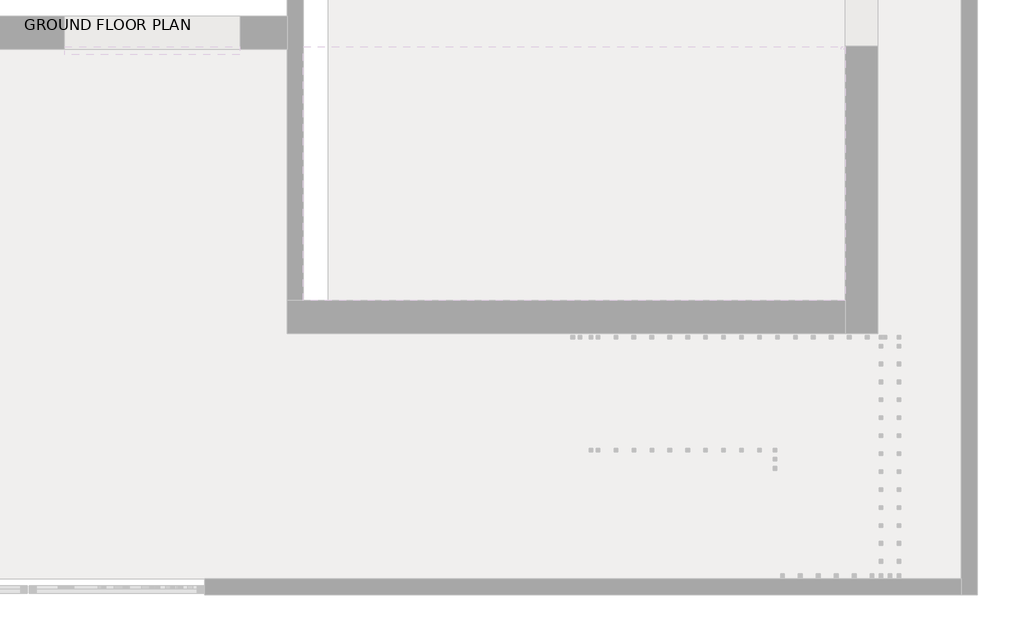
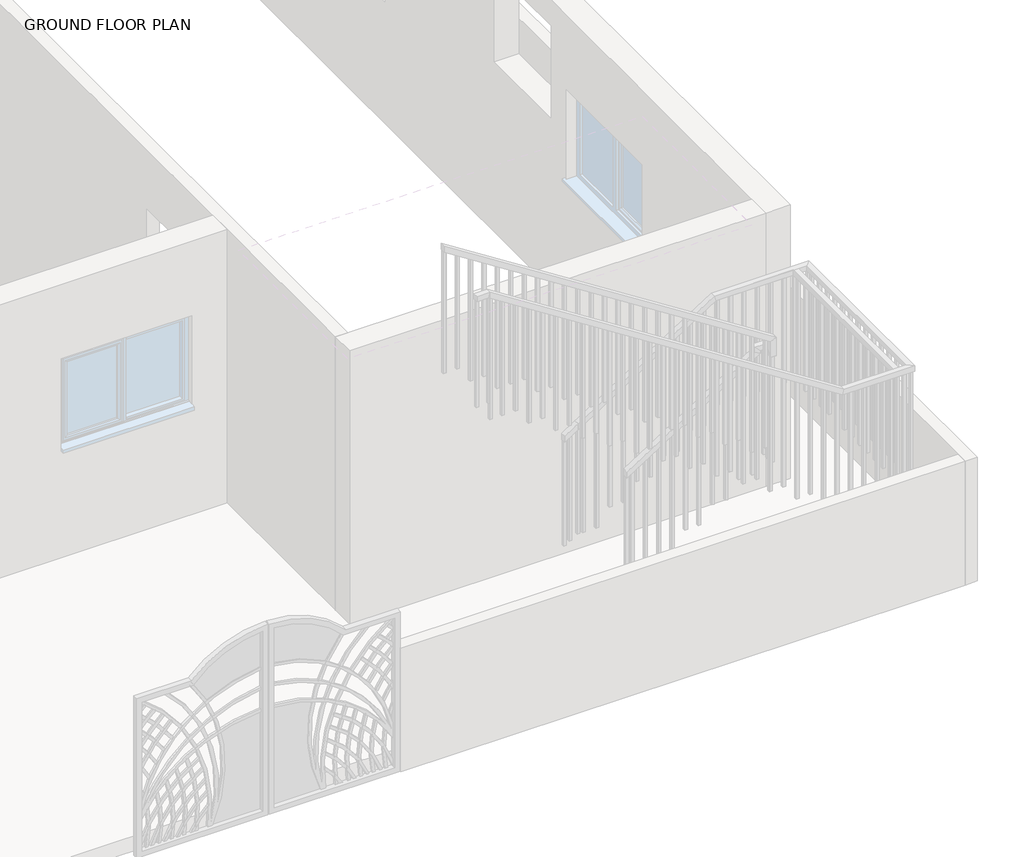
# One storey, part 10 of 23: 2 railings.
"""IFC4 building model written with IfcOpenShell, lengths in millimetres."""

from ifc_helpers import new_model, si_unit, frame, origin, place, context, project, spatial, polyline, outline, extrude, faceted_brep, element, save

model = new_model("IFC4")

# Units and contexts
model_context = context("Model", 3, world=origin())
ifc_project = project(units=[si_unit("LENGTHUNIT", "METRE", prefix="MILLI")], contexts=[model_context])

# Site, building, storey
site = spatial("IfcSite", under=ifc_project)
building = spatial("IfcBuilding", under=site)
storey = spatial("IfcBuildingStorey", under=building, Name="GROUND FLOOR PLAN", Elevation=487.68)

# Railings
placement = place(None, origin())
element("IfcRailing", 1, ObjectType="1100mm", at=placement, inside=storey, context=model_context, shape_type="SolidModel", body=[
    faceted_brep([(-8680.149573, -10220.0521308, 1912.8), (-8680.149573, -10220.0521308, 1853.4423995), (-8680.149573, -10270.0521308, 1853.4423995), (-8680.149573, -10270.0521308, 1912.8), (-7409.7306254, -10220.0521308, 2725.6), (-7395.1045513, -10220.0521308, 2675.6), (-7395.1045513, -10270.0521308, 2675.6), (-7409.7306254, -10270.0521308, 2725.6), (-6495.8132565, -10220.0521308, 2725.6), (-6495.8132565, -10220.0521308, 2675.6), (-6545.8132565, -10270.0521308, 2675.6), (-6545.8132565, -10270.0521308, 2725.6), (-6495.8132565, -11933.6860066, 2725.6), (-6495.8132565, -11933.6860066, 2675.6), (-6545.8132565, -11883.6860066, 2675.6), (-6545.8132565, -11883.6860066, 2725.6), (-7155.718398, -11933.6860066, 2725.6), (-7170.3479429, -11933.6860066, 2675.6), (-7170.3479429, -11883.6860066, 2675.6), (-7155.718398, -11883.6860066, 2725.6), (-10457.8773536, -11933.6860066, 4838.88), (-10457.8773536, -11883.6860066, 4838.88), (-10457.8773536, -11883.6860066, 4779.517542), (-10457.8773536, -11933.6860066, 4779.517542)], [[[0, 1, 2, 3]], [[1, 0, 4, 5]], [[2, 1, 5, 6]], [[3, 2, 6, 7]], [[0, 3, 7, 4]], [[5, 4, 8, 9]], [[6, 5, 9, 10]], [[7, 6, 10, 11]], [[4, 7, 11, 8]], [[9, 8, 12, 13]], [[10, 9, 13, 14]], [[11, 10, 14, 15]], [[8, 11, 15, 12]], [[13, 12, 16, 17]], [[14, 13, 17, 18]], [[15, 14, 18, 19]], [[12, 15, 19, 16]], [[20, 21, 22, 23]], [[17, 16, 20, 23]], [[18, 17, 23, 22]], [[19, 18, 22, 21]], [[16, 19, 21, 20]]]),
    extrude(outline(polyline([(4691.8007425, -10320.8132565), (4707.7999723, -10345.8132565), (3576.32, -10345.8132565), (3576.32, -10320.8132565), (4691.8007425, -10320.8132565)])), frame((0.0, -11921.1860066, 0.0), z_axis=(0.0, 1.0, 0.0), x_axis=(0.0, 0.0, 1.0)), (0.0, 0.0, 1.0), 25.0),
    extrude(outline(polyline([(4611.8045935, -10195.8132565), (4627.8038233, -10220.8132565), (3576.32, -10220.8132565), (3576.32, -10195.8132565), (4611.8045935, -10195.8132565)])), frame((0.0, -11921.1860066, 0.0), z_axis=(0.0, 1.0, 0.0), x_axis=(0.0, 0.0, 1.0)), (0.0, 0.0, 1.0), 25.0),
    extrude(outline(polyline([(4531.8084444, -10070.8132565), (4547.8076742, -10095.8132565), (3413.76, -10095.8132565), (3413.76, -10070.8132565), (4531.8084444, -10070.8132565)])), frame((0.0, -11921.1860066, 0.0), z_axis=(0.0, 1.0, 0.0), x_axis=(0.0, 0.0, 1.0)), (0.0, 0.0, 1.0), 25.0),
    extrude(outline(polyline([(4451.8122954, -9945.8132565), (4467.8115252, -9970.8132565), (3413.76, -9970.8132565), (3413.76, -9945.8132565), (4451.8122954, -9945.8132565)])), frame((0.0, -11921.1860066, 0.0), z_axis=(0.0, 1.0, 0.0), x_axis=(0.0, 0.0, 1.0)), (0.0, 0.0, 1.0), 25.0),
    extrude(outline(polyline([(4371.8161463, -9820.8132565), (4387.8153761, -9845.8132565), (3251.2, -9845.8132565), (3251.2, -9820.8132565), (4371.8161463, -9820.8132565)])), frame((0.0, -11921.1860066, 0.0), z_axis=(0.0, 1.0, 0.0), x_axis=(0.0, 0.0, 1.0)), (0.0, 0.0, 1.0), 25.0),
    extrude(outline(polyline([(4291.8423995, -9695.8132565), (4307.8371231, -9720.8132565), (3251.2, -9720.8132565), (3251.2, -9695.8132565), (4291.8423995, -9695.8132565)])), frame((0.0, -11921.1860066, 0.0), z_axis=(0.0, 1.0, 0.0), x_axis=(0.0, 0.0, 1.0)), (0.0, 0.0, 1.0), 25.0),
    extrude(outline(polyline([(4211.8238482, -9570.8132565), (4227.823078, -9595.8132565), (3088.64, -9595.8132565), (3088.64, -9570.8132565), (4211.8238482, -9570.8132565)])), frame((0.0, -11921.1860066, 0.0), z_axis=(0.0, 1.0, 0.0), x_axis=(0.0, 0.0, 1.0)), (0.0, 0.0, 1.0), 25.0),
    extrude(outline(polyline([(4131.8276992, -9445.8132565), (4147.826929, -9470.8132565), (3088.64, -9470.8132565), (3088.64, -9445.8132565), (4131.8276992, -9445.8132565)])), frame((0.0, -11921.1860066, 0.0), z_axis=(0.0, 1.0, 0.0), x_axis=(0.0, 0.0, 1.0)), (0.0, 0.0, 1.0), 25.0),
    extrude(outline(polyline([(4051.8315501, -9320.8132565), (4067.8307799, -9345.8132565), (2926.08, -9345.8132565), (2926.08, -9320.8132565), (4051.8315501, -9320.8132565)])), frame((0.0, -11921.1860066, 0.0), z_axis=(0.0, 1.0, 0.0), x_axis=(0.0, 0.0, 1.0)), (0.0, 0.0, 1.0), 25.0),
    extrude(outline(polyline([(3971.835401, -9195.8132565), (3987.8346309, -9220.8132565), (2926.08, -9220.8132565), (2926.08, -9195.8132565), (3971.835401, -9195.8132565)])), frame((0.0, -11921.1860066, 0.0), z_axis=(0.0, 1.0, 0.0), x_axis=(0.0, 0.0, 1.0)), (0.0, 0.0, 1.0), 25.0),
    extrude(outline(polyline([(3891.839252, -9070.8132565), (3907.8384818, -9095.8132565), (2763.52, -9095.8132565), (2763.52, -9070.8132565), (3891.839252, -9070.8132565)])), frame((0.0, -11921.1860066, 0.0), z_axis=(0.0, 1.0, 0.0), x_axis=(0.0, 0.0, 1.0)), (0.0, 0.0, 1.0), 25.0),
    extrude(outline(polyline([(3811.8431029, -8945.8132565), (3827.8423328, -8970.8132565), (2763.52, -8970.8132565), (2763.52, -8945.8132565), (3811.8431029, -8945.8132565)])), frame((0.0, -11921.1860066, 0.0), z_axis=(0.0, 1.0, 0.0), x_axis=(0.0, 0.0, 1.0)), (0.0, 0.0, 1.0), 25.0),
    extrude(outline(polyline([(3731.8469539, -8820.8132565), (3747.8461837, -8845.8132565), (2600.96, -8845.8132565), (2600.96, -8820.8132565), (3731.8469539, -8820.8132565)])), frame((0.0, -11921.1860066, 0.0), z_axis=(0.0, 1.0, 0.0), x_axis=(0.0, 0.0, 1.0)), (0.0, 0.0, 1.0), 25.0),
    extrude(outline(polyline([(3651.8508048, -8695.8132565), (3667.8500347, -8720.8132565), (2600.96, -8720.8132565), (2600.96, -8695.8132565), (3651.8508048, -8695.8132565)])), frame((0.0, -11921.1860066, 0.0), z_axis=(0.0, 1.0, 0.0), x_axis=(0.0, 0.0, 1.0)), (0.0, 0.0, 1.0), 25.0),
    extrude(outline(polyline([(3571.8546558, -8570.8132565), (3587.8538856, -8595.8132565), (2438.4, -8595.8132565), (2438.4, -8570.8132565), (3571.8546558, -8570.8132565)])), frame((0.0, -11921.1860066, 0.0), z_axis=(0.0, 1.0, 0.0), x_axis=(0.0, 0.0, 1.0)), (0.0, 0.0, 1.0), 25.0),
    extrude(outline(polyline([(3491.8585067, -8445.8132565), (3507.8577365, -8470.8132565), (2438.4, -8470.8132565), (2438.4, -8445.8132565), (3491.8585067, -8445.8132565)])), frame((0.0, -11921.1860066, 0.0), z_axis=(0.0, 1.0, 0.0), x_axis=(0.0, 0.0, 1.0)), (0.0, 0.0, 1.0), 25.0),
    extrude(outline(polyline([(3411.8623577, -8320.8132565), (3427.8615875, -8345.8132565), (2275.84, -8345.8132565), (2275.84, -8320.8132565), (3411.8623577, -8320.8132565)])), frame((0.0, -11921.1860066, 0.0), z_axis=(0.0, 1.0, 0.0), x_axis=(0.0, 0.0, 1.0)), (0.0, 0.0, 1.0), 25.0),
    extrude(outline(polyline([(3331.8662086, -8195.8132565), (3347.8654384, -8220.8132565), (2275.84, -8220.8132565), (2275.84, -8195.8132565), (3331.8662086, -8195.8132565)])), frame((0.0, -11921.1860066, 0.0), z_axis=(0.0, 1.0, 0.0), x_axis=(0.0, 0.0, 1.0)), (0.0, 0.0, 1.0), 25.0),
    extrude(outline(polyline([(3251.8700596, -8070.8132565), (3267.8692894, -8095.8132565), (2113.28, -8095.8132565), (2113.28, -8070.8132565), (3251.8700596, -8070.8132565)])), frame((0.0, -11921.1860066, 0.0), z_axis=(0.0, 1.0, 0.0), x_axis=(0.0, 0.0, 1.0)), (0.0, 0.0, 1.0), 25.0),
    extrude(outline(polyline([(3171.8739105, -7945.8132565), (3187.8731403, -7970.8132565), (2113.28, -7970.8132565), (2113.28, -7945.8132565), (3171.8739105, -7945.8132565)])), frame((0.0, -11921.1860066, 0.0), z_axis=(0.0, 1.0, 0.0), x_axis=(0.0, 0.0, 1.0)), (0.0, 0.0, 1.0), 25.0),
    extrude(outline(polyline([(3091.8777615, -7820.8132565), (3107.8769913, -7845.8132565), (1950.72, -7845.8132565), (1950.72, -7820.8132565), (3091.8777615, -7820.8132565)])), frame((0.0, -11921.1860066, 0.0), z_axis=(0.0, 1.0, 0.0), x_axis=(0.0, 0.0, 1.0)), (0.0, 0.0, 1.0), 25.0),
    extrude(outline(polyline([(3011.8816124, -7695.8132565), (3027.8808422, -7720.8132565), (1950.72, -7720.8132565), (1950.72, -7695.8132565), (3011.8816124, -7695.8132565)])), frame((0.0, -11921.1860066, 0.0), z_axis=(0.0, 1.0, 0.0), x_axis=(0.0, 0.0, 1.0)), (0.0, 0.0, 1.0), 25.0),
    extrude(outline(polyline([(2931.8854634, -7570.8132565), (2947.8846932, -7595.8132565), (1788.16, -7595.8132565), (1788.16, -7570.8132565), (2931.8854634, -7570.8132565)])), frame((0.0, -11921.1860066, 0.0), z_axis=(0.0, 1.0, 0.0), x_axis=(0.0, 0.0, 1.0)), (0.0, 0.0, 1.0), 25.0),
    extrude(outline(polyline([(2851.8893143, -7445.8132565), (2867.8885441, -7470.8132565), (1788.16, -7470.8132565), (1788.16, -7445.8132565), (2851.8893143, -7445.8132565)])), frame((0.0, -11921.1860066, 0.0), z_axis=(0.0, 1.0, 0.0), x_axis=(0.0, 0.0, 1.0)), (0.0, 0.0, 1.0), 25.0),
    extrude(outline(polyline([(2771.8931653, -7320.8132565), (2787.8923951, -7345.8132565), (1625.6, -7345.8132565), (1625.6, -7320.8132565), (2771.8931653, -7320.8132565)])), frame((0.0, -11921.1860066, 0.0), z_axis=(0.0, 1.0, 0.0), x_axis=(0.0, 0.0, 1.0)), (0.0, 0.0, 1.0), 25.0),
    extrude(outline(polyline([(2691.8970162, -7195.8132565), (2707.896246, -7220.8132565), (1625.6, -7220.8132565), (1625.6, -7195.8132565), (2691.8970162, -7195.8132565)])), frame((0.0, -11921.1860066, 0.0), z_axis=(0.0, 1.0, 0.0), x_axis=(0.0, 0.0, 1.0)), (0.0, 0.0, 1.0), 25.0),
    extrude(outline(polyline([(-7070.8132565, -11921.1860066), (-7095.8132565, -11921.1860066), (-7095.8132565, -11896.1860066), (-7070.8132565, -11896.1860066), (-7070.8132565, -11921.1860066)])), frame((0.0, 0.0, 1625.6), z_axis=(0.0, 0.0, 1.0), x_axis=(1.0, 0.0, 0.0)), (0.0, 0.0, 1.0), 1050.0),
    extrude(outline(polyline([(-6945.8132565, -11921.1860066), (-6970.8132565, -11921.1860066), (-6970.8132565, -11896.1860066), (-6945.8132565, -11896.1860066), (-6945.8132565, -11921.1860066)])), frame((0.0, 0.0, 1625.6), z_axis=(0.0, 0.0, 1.0), x_axis=(1.0, 0.0, 0.0)), (0.0, 0.0, 1.0), 1050.0),
    extrude(outline(polyline([(-6820.8132565, -11921.1860066), (-6845.8132565, -11921.1860066), (-6845.8132565, -11896.1860066), (-6820.8132565, -11896.1860066), (-6820.8132565, -11921.1860066)])), frame((0.0, 0.0, 1625.6), z_axis=(0.0, 0.0, 1.0), x_axis=(1.0, 0.0, 0.0)), (0.0, 0.0, 1.0), 1050.0),
    extrude(outline(polyline([(-6695.8132565, -11921.1860066), (-6720.8132565, -11921.1860066), (-6720.8132565, -11896.1860066), (-6695.8132565, -11896.1860066), (-6695.8132565, -11921.1860066)])), frame((0.0, 0.0, 1625.6), z_axis=(0.0, 0.0, 1.0), x_axis=(1.0, 0.0, 0.0)), (0.0, 0.0, 1.0), 1050.0),
    extrude(outline(polyline([(-6570.8132565, -11921.1860066), (-6595.8132565, -11921.1860066), (-6595.8132565, -11896.1860066), (-6570.8132565, -11896.1860066), (-6570.8132565, -11921.1860066)])), frame((0.0, 0.0, 1625.6), z_axis=(0.0, 0.0, 1.0), x_axis=(1.0, 0.0, 0.0)), (0.0, 0.0, 1.0), 1050.0),
    extrude(outline(polyline([(-6508.3132565, -11795.0521308), (-6508.3132565, -11820.0521308), (-6533.3132565, -11820.0521308), (-6533.3132565, -11795.0521308), (-6508.3132565, -11795.0521308)])), frame((0.0, 0.0, 1625.6), z_axis=(0.0, 0.0, 1.0), x_axis=(1.0, 0.0, 0.0)), (0.0, 0.0, 1.0), 1050.0),
    extrude(outline(polyline([(-6508.3132565, -11670.0521308), (-6508.3132565, -11695.0521308), (-6533.3132565, -11695.0521308), (-6533.3132565, -11670.0521308), (-6508.3132565, -11670.0521308)])), frame((0.0, 0.0, 1625.6), z_axis=(0.0, 0.0, 1.0), x_axis=(1.0, 0.0, 0.0)), (0.0, 0.0, 1.0), 1050.0),
    extrude(outline(polyline([(-6508.3132565, -11545.0521308), (-6508.3132565, -11570.0521308), (-6533.3132565, -11570.0521308), (-6533.3132565, -11545.0521308), (-6508.3132565, -11545.0521308)])), frame((0.0, 0.0, 1625.6), z_axis=(0.0, 0.0, 1.0), x_axis=(1.0, 0.0, 0.0)), (0.0, 0.0, 1.0), 1050.0),
    extrude(outline(polyline([(-6508.3132565, -11420.0521308), (-6508.3132565, -11445.0521308), (-6533.3132565, -11445.0521308), (-6533.3132565, -11420.0521308), (-6508.3132565, -11420.0521308)])), frame((0.0, 0.0, 1625.6), z_axis=(0.0, 0.0, 1.0), x_axis=(1.0, 0.0, 0.0)), (0.0, 0.0, 1.0), 1050.0),
    extrude(outline(polyline([(-6508.3132565, -11295.0521308), (-6508.3132565, -11320.0521308), (-6533.3132565, -11320.0521308), (-6533.3132565, -11295.0521308), (-6508.3132565, -11295.0521308)])), frame((0.0, 0.0, 1625.6), z_axis=(0.0, 0.0, 1.0), x_axis=(1.0, 0.0, 0.0)), (0.0, 0.0, 1.0), 1050.0),
    extrude(outline(polyline([(-6508.3132565, -11170.0521308), (-6508.3132565, -11195.0521308), (-6533.3132565, -11195.0521308), (-6533.3132565, -11170.0521308), (-6508.3132565, -11170.0521308)])), frame((0.0, 0.0, 1625.6), z_axis=(0.0, 0.0, 1.0), x_axis=(1.0, 0.0, 0.0)), (0.0, 0.0, 1.0), 1050.0),
    extrude(outline(polyline([(-6508.3132565, -11045.0521308), (-6508.3132565, -11070.0521308), (-6533.3132565, -11070.0521308), (-6533.3132565, -11045.0521308), (-6508.3132565, -11045.0521308)])), frame((0.0, 0.0, 1625.6), z_axis=(0.0, 0.0, 1.0), x_axis=(1.0, 0.0, 0.0)), (0.0, 0.0, 1.0), 1050.0),
    extrude(outline(polyline([(-6508.3132565, -10920.0521308), (-6508.3132565, -10945.0521308), (-6533.3132565, -10945.0521308), (-6533.3132565, -10920.0521308), (-6508.3132565, -10920.0521308)])), frame((0.0, 0.0, 1625.6), z_axis=(0.0, 0.0, 1.0), x_axis=(1.0, 0.0, 0.0)), (0.0, 0.0, 1.0), 1050.0),
    extrude(outline(polyline([(-6508.3132565, -10795.0521308), (-6508.3132565, -10820.0521308), (-6533.3132565, -10820.0521308), (-6533.3132565, -10795.0521308), (-6508.3132565, -10795.0521308)])), frame((0.0, 0.0, 1625.6), z_axis=(0.0, 0.0, 1.0), x_axis=(1.0, 0.0, 0.0)), (0.0, 0.0, 1.0), 1050.0),
    extrude(outline(polyline([(-6508.3132565, -10670.0521308), (-6508.3132565, -10695.0521308), (-6533.3132565, -10695.0521308), (-6533.3132565, -10670.0521308), (-6508.3132565, -10670.0521308)])), frame((0.0, 0.0, 1625.6), z_axis=(0.0, 0.0, 1.0), x_axis=(1.0, 0.0, 0.0)), (0.0, 0.0, 1.0), 1050.0),
    extrude(outline(polyline([(-6508.3132565, -10545.0521308), (-6508.3132565, -10570.0521308), (-6533.3132565, -10570.0521308), (-6533.3132565, -10545.0521308), (-6508.3132565, -10545.0521308)])), frame((0.0, 0.0, 1625.6), z_axis=(0.0, 0.0, 1.0), x_axis=(1.0, 0.0, 0.0)), (0.0, 0.0, 1.0), 1050.0),
    extrude(outline(polyline([(-6508.3132565, -10420.0521308), (-6508.3132565, -10445.0521308), (-6533.3132565, -10445.0521308), (-6533.3132565, -10420.0521308), (-6508.3132565, -10420.0521308)])), frame((0.0, 0.0, 1625.6), z_axis=(0.0, 0.0, 1.0), x_axis=(1.0, 0.0, 0.0)), (0.0, 0.0, 1.0), 1050.0),
    extrude(outline(polyline([(-6508.3132565, -10295.0521308), (-6508.3132565, -10320.0521308), (-6533.3132565, -10320.0521308), (-6533.3132565, -10295.0521308), (-6508.3132565, -10295.0521308)])), frame((0.0, 0.0, 1625.6), z_axis=(0.0, 0.0, 1.0), x_axis=(1.0, 0.0, 0.0)), (0.0, 0.0, 1.0), 1050.0),
    extrude(outline(polyline([(-6630.149573, -10232.5521308), (-6605.149573, -10232.5521308), (-6605.149573, -10257.5521308), (-6630.149573, -10257.5521308), (-6630.149573, -10232.5521308)])), frame((0.0, 0.0, 1625.6), z_axis=(0.0, 0.0, 1.0), x_axis=(1.0, 0.0, 0.0)), (0.0, 0.0, 1.0), 1050.0),
    extrude(outline(polyline([(-6755.149573, -10232.5521308), (-6730.149573, -10232.5521308), (-6730.149573, -10257.5521308), (-6755.149573, -10257.5521308), (-6755.149573, -10232.5521308)])), frame((0.0, 0.0, 1625.6), z_axis=(0.0, 0.0, 1.0), x_axis=(1.0, 0.0, 0.0)), (0.0, 0.0, 1.0), 1050.0),
    extrude(outline(polyline([(-6880.149573, -10232.5521308), (-6855.149573, -10232.5521308), (-6855.149573, -10257.5521308), (-6880.149573, -10257.5521308), (-6880.149573, -10232.5521308)])), frame((0.0, 0.0, 1625.6), z_axis=(0.0, 0.0, 1.0), x_axis=(1.0, 0.0, 0.0)), (0.0, 0.0, 1.0), 1050.0),
    extrude(outline(polyline([(-7005.149573, -10232.5521308), (-6980.149573, -10232.5521308), (-6980.149573, -10257.5521308), (-7005.149573, -10257.5521308), (-7005.149573, -10232.5521308)])), frame((0.0, 0.0, 1625.6), z_axis=(0.0, 0.0, 1.0), x_axis=(1.0, 0.0, 0.0)), (0.0, 0.0, 1.0), 1050.0),
    extrude(outline(polyline([(-7130.149573, -10232.5521308), (-7105.149573, -10232.5521308), (-7105.149573, -10257.5521308), (-7130.149573, -10257.5521308), (-7130.149573, -10232.5521308)])), frame((0.0, 0.0, 1625.6), z_axis=(0.0, 0.0, 1.0), x_axis=(1.0, 0.0, 0.0)), (0.0, 0.0, 1.0), 1050.0),
    extrude(outline(polyline([(-7255.149573, -10232.5521308), (-7230.149573, -10232.5521308), (-7230.149573, -10257.5521308), (-7255.149573, -10257.5521308), (-7255.149573, -10232.5521308)])), frame((0.0, 0.0, 1625.6), z_axis=(0.0, 0.0, 1.0), x_axis=(1.0, 0.0, 0.0)), (0.0, 0.0, 1.0), 1050.0),
    extrude(outline(polyline([(-7380.149573, -10232.5521308), (-7355.149573, -10232.5521308), (-7355.149573, -10257.5521308), (-7380.149573, -10257.5521308), (-7380.149573, -10232.5521308)])), frame((0.0, 0.0, 1625.6), z_axis=(0.0, 0.0, 1.0), x_axis=(1.0, 0.0, 0.0)), (0.0, 0.0, 1.0), 1050.0),
    extrude(outline(polyline([(1463.04, -7505.149573), (1463.04, -7480.149573), (2621.1891352, -7480.149573), (2605.1944115, -7505.149573), (1463.04, -7505.149573)])), frame((0.0, -10257.5521308, 0.0), z_axis=(0.0, 1.0, 0.0), x_axis=(0.0, 0.0, 1.0)), (0.0, 0.0, 1.0), 25.0),
    extrude(outline(polyline([(1463.04, -7630.149573), (1463.04, -7605.149573), (2541.2155169, -7605.149573), (2525.2207932, -7630.149573), (1463.04, -7630.149573)])), frame((0.0, -10257.5521308, 0.0), z_axis=(0.0, 1.0, 0.0), x_axis=(0.0, 0.0, 1.0)), (0.0, 0.0, 1.0), 25.0),
    extrude(outline(polyline([(1300.48, -7755.149573), (1300.48, -7730.149573), (2461.2418986, -7730.149573), (2445.2471749, -7755.149573), (1300.48, -7755.149573)])), frame((0.0, -10257.5521308, 0.0), z_axis=(0.0, 1.0, 0.0), x_axis=(0.0, 0.0, 1.0)), (0.0, 0.0, 1.0), 25.0),
    extrude(outline(polyline([(1300.48, -7880.149573), (1300.48, -7855.149573), (2381.2682803, -7855.149573), (2365.2735566, -7880.149573), (1300.48, -7880.149573)])), frame((0.0, -10257.5521308, 0.0), z_axis=(0.0, 1.0, 0.0), x_axis=(0.0, 0.0, 1.0)), (0.0, 0.0, 1.0), 25.0),
    extrude(outline(polyline([(1137.92, -8005.149573), (1137.92, -7980.149573), (2301.294662, -7980.149573), (2285.2999383, -8005.149573), (1137.92, -8005.149573)])), frame((0.0, -10257.5521308, 0.0), z_axis=(0.0, 1.0, 0.0), x_axis=(0.0, 0.0, 1.0)), (0.0, 0.0, 1.0), 25.0),
    extrude(outline(polyline([(1137.92, -8130.149573), (1137.92, -8105.149573), (2221.3210437, -8105.149573), (2205.32632, -8130.149573), (1137.92, -8130.149573)])), frame((0.0, -10257.5521308, 0.0), z_axis=(0.0, 1.0, 0.0), x_axis=(0.0, 0.0, 1.0)), (0.0, 0.0, 1.0), 25.0),
    extrude(outline(polyline([(975.36, -8255.149573), (975.36, -8230.149573), (2141.3474254, -8230.149573), (2125.3527017, -8255.149573), (975.36, -8255.149573)])), frame((0.0, -10257.5521308, 0.0), z_axis=(0.0, 1.0, 0.0), x_axis=(0.0, 0.0, 1.0)), (0.0, 0.0, 1.0), 25.0),
    extrude(outline(polyline([(975.36, -8380.149573), (975.36, -8355.149573), (2061.3738071, -8355.149573), (2045.3790834, -8380.149573), (975.36, -8380.149573)])), frame((0.0, -10257.5521308, 0.0), z_axis=(0.0, 1.0, 0.0), x_axis=(0.0, 0.0, 1.0)), (0.0, 0.0, 1.0), 25.0),
    extrude(outline(polyline([(812.8, -8505.149573), (812.8, -8480.149573), (1981.4001888, -8480.149573), (1965.4054651, -8505.149573), (812.8, -8505.149573)])), frame((0.0, -10257.5521308, 0.0), z_axis=(0.0, 1.0, 0.0), x_axis=(0.0, 0.0, 1.0)), (0.0, 0.0, 1.0), 25.0),
    extrude(outline(polyline([(812.8, -8630.149573), (812.8, -8605.149573), (1901.4265705, -8605.149573), (1885.4318468, -8630.149573), (812.8, -8630.149573)])), frame((0.0, -10257.5521308, 0.0), z_axis=(0.0, 1.0, 0.0), x_axis=(0.0, 0.0, 1.0)), (0.0, 0.0, 1.0), 25.0),
    extrude(outline(polyline([(-6508.3132565, -11896.1860066), (-6508.3132565, -11921.1860066), (-6533.3132565, -11921.1860066), (-6533.3132565, -11896.1860066), (-6508.3132565, -11896.1860066)])), frame((0.0, 0.0, 1625.6), z_axis=(0.0, 0.0, 1.0), x_axis=(1.0, 0.0, 0.0)), (0.0, 0.0, 1.0), 1050.0),
    extrude(outline(polyline([(-6533.3132565, -10232.5521308), (-6508.3132565, -10232.5521308), (-6508.3132565, -10257.5521308), (-6533.3132565, -10257.5521308), (-6533.3132565, -10232.5521308)])), frame((0.0, 0.0, 1625.6), z_axis=(0.0, 0.0, 1.0), x_axis=(1.0, 0.0, 0.0)), (0.0, 0.0, 1.0), 1050.0),
    extrude(outline(polyline([(4763.5183122, -10432.8773536), (4779.517542, -10457.8773536), (3576.32, -10457.8773536), (3576.32, -10432.8773536), (4763.5183122, -10432.8773536)])), frame((0.0, -11921.1860066, 0.0), z_axis=(0.0, 1.0, 0.0), x_axis=(0.0, 0.0, 1.0)), (0.0, 0.0, 1.0), 25.0),
    extrude(outline(polyline([(812.8, -8680.149573), (812.8, -8655.149573), (1869.4371231, -8655.149573), (1853.4423995, -8680.149573), (812.8, -8680.149573)])), frame((0.0, -10257.5521308, 0.0), z_axis=(0.0, 1.0, 0.0), x_axis=(0.0, 0.0, 1.0)), (0.0, 0.0, 1.0), 25.0),
])
element("IfcRailing", 2, ObjectType="1100mm", at=placement, inside=storey, context=model_context, shape_type="SolidModel", body=[
    faceted_brep([(-8680.149573, -10220.0521308, 1912.8), (-8680.149573, -10220.0521308, 1853.4423995), (-8680.149573, -10270.0521308, 1853.4423995), (-8680.149573, -10270.0521308, 1912.8), (-7409.7306254, -10220.0521308, 2725.6), (-7395.1045513, -10220.0521308, 2675.6), (-7395.1045513, -10270.0521308, 2675.6), (-7409.7306254, -10270.0521308, 2725.6), (-6495.8132565, -10220.0521308, 2725.6), (-6495.8132565, -10220.0521308, 2675.6), (-6545.8132565, -10270.0521308, 2675.6), (-6545.8132565, -10270.0521308, 2725.6), (-6495.8132565, -11933.6860066, 2725.6), (-6495.8132565, -11933.6860066, 2675.6), (-6545.8132565, -11883.6860066, 2675.6), (-6545.8132565, -11883.6860066, 2725.6), (-7155.718398, -11933.6860066, 2725.6), (-7170.3479429, -11933.6860066, 2675.6), (-7170.3479429, -11883.6860066, 2675.6), (-7155.718398, -11883.6860066, 2725.6), (-10457.8773536, -11933.6860066, 4838.88), (-10457.8773536, -11883.6860066, 4838.88), (-10457.8773536, -11883.6860066, 4779.517542), (-10457.8773536, -11933.6860066, 4779.517542)], [[[0, 1, 2, 3]], [[1, 0, 4, 5]], [[2, 1, 5, 6]], [[3, 2, 6, 7]], [[0, 3, 7, 4]], [[5, 4, 8, 9]], [[6, 5, 9, 10]], [[7, 6, 10, 11]], [[4, 7, 11, 8]], [[9, 8, 12, 13]], [[10, 9, 13, 14]], [[11, 10, 14, 15]], [[8, 11, 15, 12]], [[13, 12, 16, 17]], [[14, 13, 17, 18]], [[15, 14, 18, 19]], [[12, 15, 19, 16]], [[20, 21, 22, 23]], [[17, 16, 20, 23]], [[18, 17, 23, 22]], [[19, 18, 22, 21]], [[16, 19, 21, 20]]]),
    extrude(outline(polyline([(4691.8007425, -10320.8132565), (4707.7999723, -10345.8132565), (3576.32, -10345.8132565), (3576.32, -10320.8132565), (4691.8007425, -10320.8132565)])), frame((0.0, -11921.1860066, 0.0), z_axis=(0.0, 1.0, 0.0), x_axis=(0.0, 0.0, 1.0)), (0.0, 0.0, 1.0), 25.0),
    extrude(outline(polyline([(4611.8045935, -10195.8132565), (4627.8038233, -10220.8132565), (3576.32, -10220.8132565), (3576.32, -10195.8132565), (4611.8045935, -10195.8132565)])), frame((0.0, -11921.1860066, 0.0), z_axis=(0.0, 1.0, 0.0), x_axis=(0.0, 0.0, 1.0)), (0.0, 0.0, 1.0), 25.0),
    extrude(outline(polyline([(4531.8084444, -10070.8132565), (4547.8076742, -10095.8132565), (3413.76, -10095.8132565), (3413.76, -10070.8132565), (4531.8084444, -10070.8132565)])), frame((0.0, -11921.1860066, 0.0), z_axis=(0.0, 1.0, 0.0), x_axis=(0.0, 0.0, 1.0)), (0.0, 0.0, 1.0), 25.0),
    extrude(outline(polyline([(4451.8122954, -9945.8132565), (4467.8115252, -9970.8132565), (3413.76, -9970.8132565), (3413.76, -9945.8132565), (4451.8122954, -9945.8132565)])), frame((0.0, -11921.1860066, 0.0), z_axis=(0.0, 1.0, 0.0), x_axis=(0.0, 0.0, 1.0)), (0.0, 0.0, 1.0), 25.0),
    extrude(outline(polyline([(4371.8161463, -9820.8132565), (4387.8153761, -9845.8132565), (3251.2, -9845.8132565), (3251.2, -9820.8132565), (4371.8161463, -9820.8132565)])), frame((0.0, -11921.1860066, 0.0), z_axis=(0.0, 1.0, 0.0), x_axis=(0.0, 0.0, 1.0)), (0.0, 0.0, 1.0), 25.0),
    extrude(outline(polyline([(4291.8423995, -9695.8132565), (4307.8371231, -9720.8132565), (3251.2, -9720.8132565), (3251.2, -9695.8132565), (4291.8423995, -9695.8132565)])), frame((0.0, -11921.1860066, 0.0), z_axis=(0.0, 1.0, 0.0), x_axis=(0.0, 0.0, 1.0)), (0.0, 0.0, 1.0), 25.0),
    extrude(outline(polyline([(4211.8238482, -9570.8132565), (4227.823078, -9595.8132565), (3088.64, -9595.8132565), (3088.64, -9570.8132565), (4211.8238482, -9570.8132565)])), frame((0.0, -11921.1860066, 0.0), z_axis=(0.0, 1.0, 0.0), x_axis=(0.0, 0.0, 1.0)), (0.0, 0.0, 1.0), 25.0),
    extrude(outline(polyline([(4131.8276992, -9445.8132565), (4147.826929, -9470.8132565), (3088.64, -9470.8132565), (3088.64, -9445.8132565), (4131.8276992, -9445.8132565)])), frame((0.0, -11921.1860066, 0.0), z_axis=(0.0, 1.0, 0.0), x_axis=(0.0, 0.0, 1.0)), (0.0, 0.0, 1.0), 25.0),
    extrude(outline(polyline([(4051.8315501, -9320.8132565), (4067.8307799, -9345.8132565), (2926.08, -9345.8132565), (2926.08, -9320.8132565), (4051.8315501, -9320.8132565)])), frame((0.0, -11921.1860066, 0.0), z_axis=(0.0, 1.0, 0.0), x_axis=(0.0, 0.0, 1.0)), (0.0, 0.0, 1.0), 25.0),
    extrude(outline(polyline([(3971.835401, -9195.8132565), (3987.8346309, -9220.8132565), (2926.08, -9220.8132565), (2926.08, -9195.8132565), (3971.835401, -9195.8132565)])), frame((0.0, -11921.1860066, 0.0), z_axis=(0.0, 1.0, 0.0), x_axis=(0.0, 0.0, 1.0)), (0.0, 0.0, 1.0), 25.0),
    extrude(outline(polyline([(3891.839252, -9070.8132565), (3907.8384818, -9095.8132565), (2763.52, -9095.8132565), (2763.52, -9070.8132565), (3891.839252, -9070.8132565)])), frame((0.0, -11921.1860066, 0.0), z_axis=(0.0, 1.0, 0.0), x_axis=(0.0, 0.0, 1.0)), (0.0, 0.0, 1.0), 25.0),
    extrude(outline(polyline([(3811.8431029, -8945.8132565), (3827.8423328, -8970.8132565), (2763.52, -8970.8132565), (2763.52, -8945.8132565), (3811.8431029, -8945.8132565)])), frame((0.0, -11921.1860066, 0.0), z_axis=(0.0, 1.0, 0.0), x_axis=(0.0, 0.0, 1.0)), (0.0, 0.0, 1.0), 25.0),
    extrude(outline(polyline([(3731.8469539, -8820.8132565), (3747.8461837, -8845.8132565), (2600.96, -8845.8132565), (2600.96, -8820.8132565), (3731.8469539, -8820.8132565)])), frame((0.0, -11921.1860066, 0.0), z_axis=(0.0, 1.0, 0.0), x_axis=(0.0, 0.0, 1.0)), (0.0, 0.0, 1.0), 25.0),
    extrude(outline(polyline([(3651.8508048, -8695.8132565), (3667.8500347, -8720.8132565), (2600.96, -8720.8132565), (2600.96, -8695.8132565), (3651.8508048, -8695.8132565)])), frame((0.0, -11921.1860066, 0.0), z_axis=(0.0, 1.0, 0.0), x_axis=(0.0, 0.0, 1.0)), (0.0, 0.0, 1.0), 25.0),
    extrude(outline(polyline([(3571.8546558, -8570.8132565), (3587.8538856, -8595.8132565), (2438.4, -8595.8132565), (2438.4, -8570.8132565), (3571.8546558, -8570.8132565)])), frame((0.0, -11921.1860066, 0.0), z_axis=(0.0, 1.0, 0.0), x_axis=(0.0, 0.0, 1.0)), (0.0, 0.0, 1.0), 25.0),
    extrude(outline(polyline([(3491.8585067, -8445.8132565), (3507.8577365, -8470.8132565), (2438.4, -8470.8132565), (2438.4, -8445.8132565), (3491.8585067, -8445.8132565)])), frame((0.0, -11921.1860066, 0.0), z_axis=(0.0, 1.0, 0.0), x_axis=(0.0, 0.0, 1.0)), (0.0, 0.0, 1.0), 25.0),
    extrude(outline(polyline([(3411.8623577, -8320.8132565), (3427.8615875, -8345.8132565), (2275.84, -8345.8132565), (2275.84, -8320.8132565), (3411.8623577, -8320.8132565)])), frame((0.0, -11921.1860066, 0.0), z_axis=(0.0, 1.0, 0.0), x_axis=(0.0, 0.0, 1.0)), (0.0, 0.0, 1.0), 25.0),
    extrude(outline(polyline([(3331.8662086, -8195.8132565), (3347.8654384, -8220.8132565), (2275.84, -8220.8132565), (2275.84, -8195.8132565), (3331.8662086, -8195.8132565)])), frame((0.0, -11921.1860066, 0.0), z_axis=(0.0, 1.0, 0.0), x_axis=(0.0, 0.0, 1.0)), (0.0, 0.0, 1.0), 25.0),
    extrude(outline(polyline([(3251.8700596, -8070.8132565), (3267.8692894, -8095.8132565), (2113.28, -8095.8132565), (2113.28, -8070.8132565), (3251.8700596, -8070.8132565)])), frame((0.0, -11921.1860066, 0.0), z_axis=(0.0, 1.0, 0.0), x_axis=(0.0, 0.0, 1.0)), (0.0, 0.0, 1.0), 25.0),
    extrude(outline(polyline([(3171.8739105, -7945.8132565), (3187.8731403, -7970.8132565), (2113.28, -7970.8132565), (2113.28, -7945.8132565), (3171.8739105, -7945.8132565)])), frame((0.0, -11921.1860066, 0.0), z_axis=(0.0, 1.0, 0.0), x_axis=(0.0, 0.0, 1.0)), (0.0, 0.0, 1.0), 25.0),
    extrude(outline(polyline([(3091.8777615, -7820.8132565), (3107.8769913, -7845.8132565), (1950.72, -7845.8132565), (1950.72, -7820.8132565), (3091.8777615, -7820.8132565)])), frame((0.0, -11921.1860066, 0.0), z_axis=(0.0, 1.0, 0.0), x_axis=(0.0, 0.0, 1.0)), (0.0, 0.0, 1.0), 25.0),
    extrude(outline(polyline([(3011.8816124, -7695.8132565), (3027.8808422, -7720.8132565), (1950.72, -7720.8132565), (1950.72, -7695.8132565), (3011.8816124, -7695.8132565)])), frame((0.0, -11921.1860066, 0.0), z_axis=(0.0, 1.0, 0.0), x_axis=(0.0, 0.0, 1.0)), (0.0, 0.0, 1.0), 25.0),
    extrude(outline(polyline([(2931.8854634, -7570.8132565), (2947.8846932, -7595.8132565), (1788.16, -7595.8132565), (1788.16, -7570.8132565), (2931.8854634, -7570.8132565)])), frame((0.0, -11921.1860066, 0.0), z_axis=(0.0, 1.0, 0.0), x_axis=(0.0, 0.0, 1.0)), (0.0, 0.0, 1.0), 25.0),
    extrude(outline(polyline([(2851.8893143, -7445.8132565), (2867.8885441, -7470.8132565), (1788.16, -7470.8132565), (1788.16, -7445.8132565), (2851.8893143, -7445.8132565)])), frame((0.0, -11921.1860066, 0.0), z_axis=(0.0, 1.0, 0.0), x_axis=(0.0, 0.0, 1.0)), (0.0, 0.0, 1.0), 25.0),
    extrude(outline(polyline([(2771.8931653, -7320.8132565), (2787.8923951, -7345.8132565), (1625.6, -7345.8132565), (1625.6, -7320.8132565), (2771.8931653, -7320.8132565)])), frame((0.0, -11921.1860066, 0.0), z_axis=(0.0, 1.0, 0.0), x_axis=(0.0, 0.0, 1.0)), (0.0, 0.0, 1.0), 25.0),
    extrude(outline(polyline([(2691.8970162, -7195.8132565), (2707.896246, -7220.8132565), (1625.6, -7220.8132565), (1625.6, -7195.8132565), (2691.8970162, -7195.8132565)])), frame((0.0, -11921.1860066, 0.0), z_axis=(0.0, 1.0, 0.0), x_axis=(0.0, 0.0, 1.0)), (0.0, 0.0, 1.0), 25.0),
    extrude(outline(polyline([(-7070.8132565, -11921.1860066), (-7095.8132565, -11921.1860066), (-7095.8132565, -11896.1860066), (-7070.8132565, -11896.1860066), (-7070.8132565, -11921.1860066)])), frame((0.0, 0.0, 1625.6), z_axis=(0.0, 0.0, 1.0), x_axis=(1.0, 0.0, 0.0)), (0.0, 0.0, 1.0), 1050.0),
    extrude(outline(polyline([(-6945.8132565, -11921.1860066), (-6970.8132565, -11921.1860066), (-6970.8132565, -11896.1860066), (-6945.8132565, -11896.1860066), (-6945.8132565, -11921.1860066)])), frame((0.0, 0.0, 1625.6), z_axis=(0.0, 0.0, 1.0), x_axis=(1.0, 0.0, 0.0)), (0.0, 0.0, 1.0), 1050.0),
    extrude(outline(polyline([(-6820.8132565, -11921.1860066), (-6845.8132565, -11921.1860066), (-6845.8132565, -11896.1860066), (-6820.8132565, -11896.1860066), (-6820.8132565, -11921.1860066)])), frame((0.0, 0.0, 1625.6), z_axis=(0.0, 0.0, 1.0), x_axis=(1.0, 0.0, 0.0)), (0.0, 0.0, 1.0), 1050.0),
    extrude(outline(polyline([(-6695.8132565, -11921.1860066), (-6720.8132565, -11921.1860066), (-6720.8132565, -11896.1860066), (-6695.8132565, -11896.1860066), (-6695.8132565, -11921.1860066)])), frame((0.0, 0.0, 1625.6), z_axis=(0.0, 0.0, 1.0), x_axis=(1.0, 0.0, 0.0)), (0.0, 0.0, 1.0), 1050.0),
    extrude(outline(polyline([(-6570.8132565, -11921.1860066), (-6595.8132565, -11921.1860066), (-6595.8132565, -11896.1860066), (-6570.8132565, -11896.1860066), (-6570.8132565, -11921.1860066)])), frame((0.0, 0.0, 1625.6), z_axis=(0.0, 0.0, 1.0), x_axis=(1.0, 0.0, 0.0)), (0.0, 0.0, 1.0), 1050.0),
    extrude(outline(polyline([(-6508.3132565, -11795.0521308), (-6508.3132565, -11820.0521308), (-6533.3132565, -11820.0521308), (-6533.3132565, -11795.0521308), (-6508.3132565, -11795.0521308)])), frame((0.0, 0.0, 1625.6), z_axis=(0.0, 0.0, 1.0), x_axis=(1.0, 0.0, 0.0)), (0.0, 0.0, 1.0), 1050.0),
    extrude(outline(polyline([(-6508.3132565, -11670.0521308), (-6508.3132565, -11695.0521308), (-6533.3132565, -11695.0521308), (-6533.3132565, -11670.0521308), (-6508.3132565, -11670.0521308)])), frame((0.0, 0.0, 1625.6), z_axis=(0.0, 0.0, 1.0), x_axis=(1.0, 0.0, 0.0)), (0.0, 0.0, 1.0), 1050.0),
    extrude(outline(polyline([(-6508.3132565, -11545.0521308), (-6508.3132565, -11570.0521308), (-6533.3132565, -11570.0521308), (-6533.3132565, -11545.0521308), (-6508.3132565, -11545.0521308)])), frame((0.0, 0.0, 1625.6), z_axis=(0.0, 0.0, 1.0), x_axis=(1.0, 0.0, 0.0)), (0.0, 0.0, 1.0), 1050.0),
    extrude(outline(polyline([(-6508.3132565, -11420.0521308), (-6508.3132565, -11445.0521308), (-6533.3132565, -11445.0521308), (-6533.3132565, -11420.0521308), (-6508.3132565, -11420.0521308)])), frame((0.0, 0.0, 1625.6), z_axis=(0.0, 0.0, 1.0), x_axis=(1.0, 0.0, 0.0)), (0.0, 0.0, 1.0), 1050.0),
    extrude(outline(polyline([(-6508.3132565, -11295.0521308), (-6508.3132565, -11320.0521308), (-6533.3132565, -11320.0521308), (-6533.3132565, -11295.0521308), (-6508.3132565, -11295.0521308)])), frame((0.0, 0.0, 1625.6), z_axis=(0.0, 0.0, 1.0), x_axis=(1.0, 0.0, 0.0)), (0.0, 0.0, 1.0), 1050.0),
    extrude(outline(polyline([(-6508.3132565, -11170.0521308), (-6508.3132565, -11195.0521308), (-6533.3132565, -11195.0521308), (-6533.3132565, -11170.0521308), (-6508.3132565, -11170.0521308)])), frame((0.0, 0.0, 1625.6), z_axis=(0.0, 0.0, 1.0), x_axis=(1.0, 0.0, 0.0)), (0.0, 0.0, 1.0), 1050.0),
    extrude(outline(polyline([(-6508.3132565, -11045.0521308), (-6508.3132565, -11070.0521308), (-6533.3132565, -11070.0521308), (-6533.3132565, -11045.0521308), (-6508.3132565, -11045.0521308)])), frame((0.0, 0.0, 1625.6), z_axis=(0.0, 0.0, 1.0), x_axis=(1.0, 0.0, 0.0)), (0.0, 0.0, 1.0), 1050.0),
    extrude(outline(polyline([(-6508.3132565, -10920.0521308), (-6508.3132565, -10945.0521308), (-6533.3132565, -10945.0521308), (-6533.3132565, -10920.0521308), (-6508.3132565, -10920.0521308)])), frame((0.0, 0.0, 1625.6), z_axis=(0.0, 0.0, 1.0), x_axis=(1.0, 0.0, 0.0)), (0.0, 0.0, 1.0), 1050.0),
    extrude(outline(polyline([(-6508.3132565, -10795.0521308), (-6508.3132565, -10820.0521308), (-6533.3132565, -10820.0521308), (-6533.3132565, -10795.0521308), (-6508.3132565, -10795.0521308)])), frame((0.0, 0.0, 1625.6), z_axis=(0.0, 0.0, 1.0), x_axis=(1.0, 0.0, 0.0)), (0.0, 0.0, 1.0), 1050.0),
    extrude(outline(polyline([(-6508.3132565, -10670.0521308), (-6508.3132565, -10695.0521308), (-6533.3132565, -10695.0521308), (-6533.3132565, -10670.0521308), (-6508.3132565, -10670.0521308)])), frame((0.0, 0.0, 1625.6), z_axis=(0.0, 0.0, 1.0), x_axis=(1.0, 0.0, 0.0)), (0.0, 0.0, 1.0), 1050.0),
    extrude(outline(polyline([(-6508.3132565, -10545.0521308), (-6508.3132565, -10570.0521308), (-6533.3132565, -10570.0521308), (-6533.3132565, -10545.0521308), (-6508.3132565, -10545.0521308)])), frame((0.0, 0.0, 1625.6), z_axis=(0.0, 0.0, 1.0), x_axis=(1.0, 0.0, 0.0)), (0.0, 0.0, 1.0), 1050.0),
    extrude(outline(polyline([(-6508.3132565, -10420.0521308), (-6508.3132565, -10445.0521308), (-6533.3132565, -10445.0521308), (-6533.3132565, -10420.0521308), (-6508.3132565, -10420.0521308)])), frame((0.0, 0.0, 1625.6), z_axis=(0.0, 0.0, 1.0), x_axis=(1.0, 0.0, 0.0)), (0.0, 0.0, 1.0), 1050.0),
    extrude(outline(polyline([(-6508.3132565, -10295.0521308), (-6508.3132565, -10320.0521308), (-6533.3132565, -10320.0521308), (-6533.3132565, -10295.0521308), (-6508.3132565, -10295.0521308)])), frame((0.0, 0.0, 1625.6), z_axis=(0.0, 0.0, 1.0), x_axis=(1.0, 0.0, 0.0)), (0.0, 0.0, 1.0), 1050.0),
    extrude(outline(polyline([(-6630.149573, -10232.5521308), (-6605.149573, -10232.5521308), (-6605.149573, -10257.5521308), (-6630.149573, -10257.5521308), (-6630.149573, -10232.5521308)])), frame((0.0, 0.0, 1625.6), z_axis=(0.0, 0.0, 1.0), x_axis=(1.0, 0.0, 0.0)), (0.0, 0.0, 1.0), 1050.0),
    extrude(outline(polyline([(-6755.149573, -10232.5521308), (-6730.149573, -10232.5521308), (-6730.149573, -10257.5521308), (-6755.149573, -10257.5521308), (-6755.149573, -10232.5521308)])), frame((0.0, 0.0, 1625.6), z_axis=(0.0, 0.0, 1.0), x_axis=(1.0, 0.0, 0.0)), (0.0, 0.0, 1.0), 1050.0),
    extrude(outline(polyline([(-6880.149573, -10232.5521308), (-6855.149573, -10232.5521308), (-6855.149573, -10257.5521308), (-6880.149573, -10257.5521308), (-6880.149573, -10232.5521308)])), frame((0.0, 0.0, 1625.6), z_axis=(0.0, 0.0, 1.0), x_axis=(1.0, 0.0, 0.0)), (0.0, 0.0, 1.0), 1050.0),
    extrude(outline(polyline([(-7005.149573, -10232.5521308), (-6980.149573, -10232.5521308), (-6980.149573, -10257.5521308), (-7005.149573, -10257.5521308), (-7005.149573, -10232.5521308)])), frame((0.0, 0.0, 1625.6), z_axis=(0.0, 0.0, 1.0), x_axis=(1.0, 0.0, 0.0)), (0.0, 0.0, 1.0), 1050.0),
    extrude(outline(polyline([(-7130.149573, -10232.5521308), (-7105.149573, -10232.5521308), (-7105.149573, -10257.5521308), (-7130.149573, -10257.5521308), (-7130.149573, -10232.5521308)])), frame((0.0, 0.0, 1625.6), z_axis=(0.0, 0.0, 1.0), x_axis=(1.0, 0.0, 0.0)), (0.0, 0.0, 1.0), 1050.0),
    extrude(outline(polyline([(-7255.149573, -10232.5521308), (-7230.149573, -10232.5521308), (-7230.149573, -10257.5521308), (-7255.149573, -10257.5521308), (-7255.149573, -10232.5521308)])), frame((0.0, 0.0, 1625.6), z_axis=(0.0, 0.0, 1.0), x_axis=(1.0, 0.0, 0.0)), (0.0, 0.0, 1.0), 1050.0),
    extrude(outline(polyline([(-7380.149573, -10232.5521308), (-7355.149573, -10232.5521308), (-7355.149573, -10257.5521308), (-7380.149573, -10257.5521308), (-7380.149573, -10232.5521308)])), frame((0.0, 0.0, 1625.6), z_axis=(0.0, 0.0, 1.0), x_axis=(1.0, 0.0, 0.0)), (0.0, 0.0, 1.0), 1050.0),
    extrude(outline(polyline([(1463.04, -7505.149573), (1463.04, -7480.149573), (2621.1891352, -7480.149573), (2605.1944115, -7505.149573), (1463.04, -7505.149573)])), frame((0.0, -10257.5521308, 0.0), z_axis=(0.0, 1.0, 0.0), x_axis=(0.0, 0.0, 1.0)), (0.0, 0.0, 1.0), 25.0),
    extrude(outline(polyline([(1463.04, -7630.149573), (1463.04, -7605.149573), (2541.2155169, -7605.149573), (2525.2207932, -7630.149573), (1463.04, -7630.149573)])), frame((0.0, -10257.5521308, 0.0), z_axis=(0.0, 1.0, 0.0), x_axis=(0.0, 0.0, 1.0)), (0.0, 0.0, 1.0), 25.0),
    extrude(outline(polyline([(1300.48, -7755.149573), (1300.48, -7730.149573), (2461.2418986, -7730.149573), (2445.2471749, -7755.149573), (1300.48, -7755.149573)])), frame((0.0, -10257.5521308, 0.0), z_axis=(0.0, 1.0, 0.0), x_axis=(0.0, 0.0, 1.0)), (0.0, 0.0, 1.0), 25.0),
    extrude(outline(polyline([(1300.48, -7880.149573), (1300.48, -7855.149573), (2381.2682803, -7855.149573), (2365.2735566, -7880.149573), (1300.48, -7880.149573)])), frame((0.0, -10257.5521308, 0.0), z_axis=(0.0, 1.0, 0.0), x_axis=(0.0, 0.0, 1.0)), (0.0, 0.0, 1.0), 25.0),
    extrude(outline(polyline([(1137.92, -8005.149573), (1137.92, -7980.149573), (2301.294662, -7980.149573), (2285.2999383, -8005.149573), (1137.92, -8005.149573)])), frame((0.0, -10257.5521308, 0.0), z_axis=(0.0, 1.0, 0.0), x_axis=(0.0, 0.0, 1.0)), (0.0, 0.0, 1.0), 25.0),
    extrude(outline(polyline([(1137.92, -8130.149573), (1137.92, -8105.149573), (2221.3210437, -8105.149573), (2205.32632, -8130.149573), (1137.92, -8130.149573)])), frame((0.0, -10257.5521308, 0.0), z_axis=(0.0, 1.0, 0.0), x_axis=(0.0, 0.0, 1.0)), (0.0, 0.0, 1.0), 25.0),
    extrude(outline(polyline([(975.36, -8255.149573), (975.36, -8230.149573), (2141.3474254, -8230.149573), (2125.3527017, -8255.149573), (975.36, -8255.149573)])), frame((0.0, -10257.5521308, 0.0), z_axis=(0.0, 1.0, 0.0), x_axis=(0.0, 0.0, 1.0)), (0.0, 0.0, 1.0), 25.0),
    extrude(outline(polyline([(975.36, -8380.149573), (975.36, -8355.149573), (2061.3738071, -8355.149573), (2045.3790834, -8380.149573), (975.36, -8380.149573)])), frame((0.0, -10257.5521308, 0.0), z_axis=(0.0, 1.0, 0.0), x_axis=(0.0, 0.0, 1.0)), (0.0, 0.0, 1.0), 25.0),
    extrude(outline(polyline([(812.8, -8505.149573), (812.8, -8480.149573), (1981.4001888, -8480.149573), (1965.4054651, -8505.149573), (812.8, -8505.149573)])), frame((0.0, -10257.5521308, 0.0), z_axis=(0.0, 1.0, 0.0), x_axis=(0.0, 0.0, 1.0)), (0.0, 0.0, 1.0), 25.0),
    extrude(outline(polyline([(812.8, -8630.149573), (812.8, -8605.149573), (1901.4265705, -8605.149573), (1885.4318468, -8630.149573), (812.8, -8630.149573)])), frame((0.0, -10257.5521308, 0.0), z_axis=(0.0, 1.0, 0.0), x_axis=(0.0, 0.0, 1.0)), (0.0, 0.0, 1.0), 25.0),
    extrude(outline(polyline([(-6508.3132565, -11896.1860066), (-6508.3132565, -11921.1860066), (-6533.3132565, -11921.1860066), (-6533.3132565, -11896.1860066), (-6508.3132565, -11896.1860066)])), frame((0.0, 0.0, 1625.6), z_axis=(0.0, 0.0, 1.0), x_axis=(1.0, 0.0, 0.0)), (0.0, 0.0, 1.0), 1050.0),
    extrude(outline(polyline([(-6533.3132565, -10232.5521308), (-6508.3132565, -10232.5521308), (-6508.3132565, -10257.5521308), (-6533.3132565, -10257.5521308), (-6533.3132565, -10232.5521308)])), frame((0.0, 0.0, 1625.6), z_axis=(0.0, 0.0, 1.0), x_axis=(1.0, 0.0, 0.0)), (0.0, 0.0, 1.0), 1050.0),
    extrude(outline(polyline([(4763.5183122, -10432.8773536), (4779.517542, -10457.8773536), (3576.32, -10457.8773536), (3576.32, -10432.8773536), (4763.5183122, -10432.8773536)])), frame((0.0, -11921.1860066, 0.0), z_axis=(0.0, 1.0, 0.0), x_axis=(0.0, 0.0, 1.0)), (0.0, 0.0, 1.0), 25.0),
    extrude(outline(polyline([(812.8, -8680.149573), (812.8, -8655.149573), (1869.4371231, -8655.149573), (1853.4423995, -8680.149573), (812.8, -8680.149573)])), frame((0.0, -10257.5521308, 0.0), z_axis=(0.0, 1.0, 0.0), x_axis=(0.0, 0.0, 1.0)), (0.0, 0.0, 1.0), 25.0),
])

save(model, "model.ifc")

# Revit data of these elements
# Type "1100mm"
#   built-in parameter 1008612 = 0.019685 (stored number, unit not read)
#   built-in parameter 1008611 = 0.019685 (stored number, unit not read)
#   built-in parameter 1008609 = 0.902231 (stored number, unit not read)
#   built-in parameter 1008604 = 0.19685 (stored number, unit not read)
#   built-in parameter 1008603 = 0.164042 (stored number, unit not read)
#   Railing Height = 3.608924 ft
#   built-in parameter 1008630 = 2
#   built-in parameter 1008610 = 2
#   built-in parameter 1008608 = 1
#   built-in parameter 1008618 = Baluster_Square : 25mm
# Elements 1, 2 (IfcRailing, "1100mm")
#   Phase Created = New Construction
